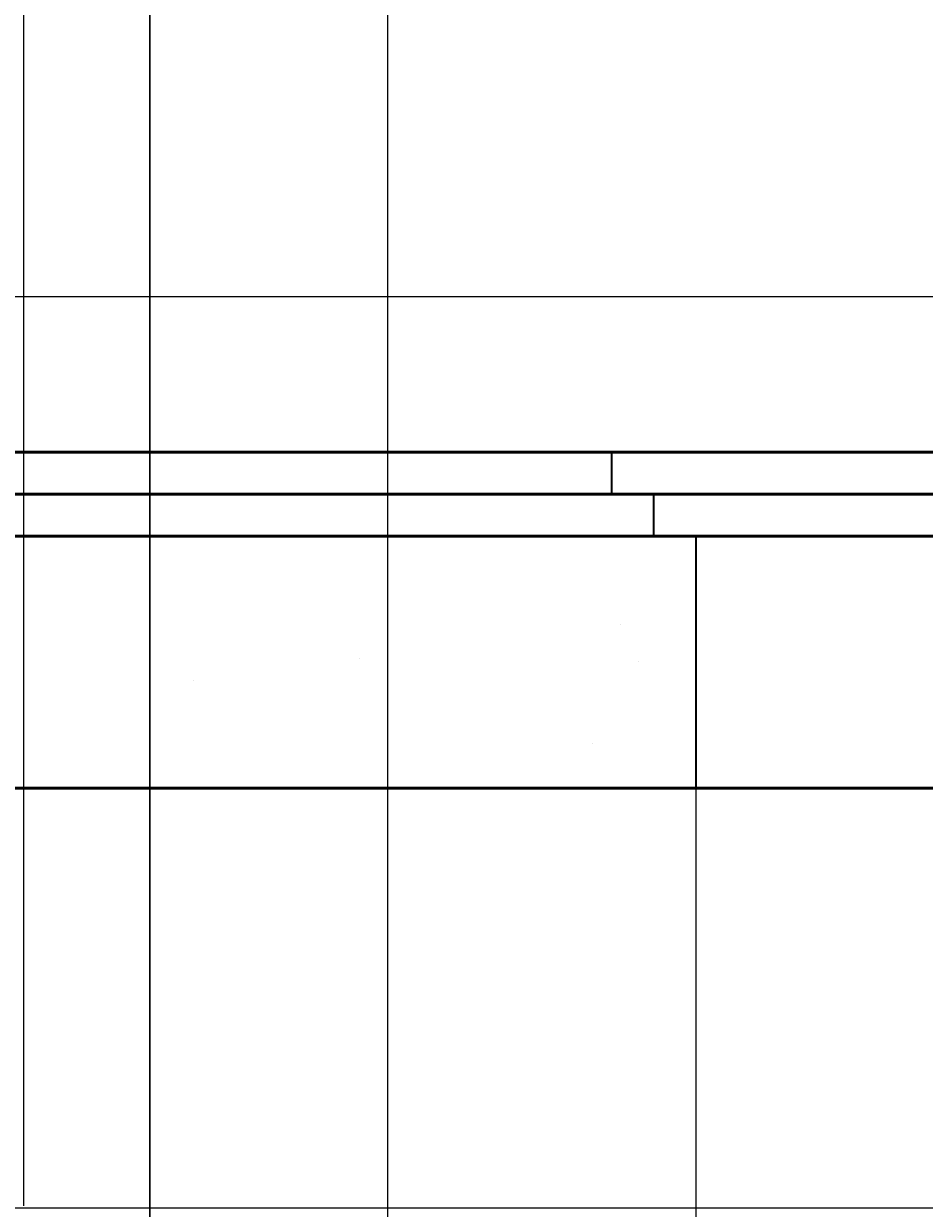
# Model space of a CAD drawing. Units: inches. Extents: x 2812 to 3051, y 1398 to 1659.
# Tile 23 of 65: x 2880 to 2902, y 1472 to 1500. Entities that reach past the tile are written whole.
import ezdxf

# ---------------------------------------------------------------- set-up
doc = ezdxf.new("R2010")
doc.units = ezdxf.units.IN
for name, color, linetype, lineweight in [('A-ANNO-DIMS', 2, 'Continuous', 18), ('S-CONC', 7, 'Continuous', 50), ('S-CONC-PATT', 8, 'Continuous', 18), ('S-CONC-SLAB', 7, 'Continuous', 35)]:
    doc.layers.add(name, color=color, linetype=linetype, lineweight=lineweight)
doc.styles.get("Standard").update_dxf_attribs({"font": 'arial.ttf'})
doc.dimstyles.get("Standard").update_dxf_attribs({"dimtxt": 0.18, "dimasz": 0.18, "dimexe": 0.18, "dimexo": 0.0625, "dimgap": 0.09, "dimtad": 0, "dimtih": 1, "dimtoh": 1, "dimdec": 4, "dimzin": 0, "dimdsep": 46, "dimtxsty": 'Standard', "dimcen": 0.09, "dimadec": 0, "dimazin": 0, "dimtfac": 1, "dimtdec": 4, "dimtofl": 0, "dimtmove": 0, "dimatfit": 3, "dimfxl": 1, "dimtolj": 1, "dimtzin": 0, "dimarcsym": 0})

# ---------------------------------------------------------------- blocks, each defined once
blk = doc.blocks.new('COVER-SLAB-PLAN')
for p, q in [((2, 7), (2, 8)), ((1, 6), (1, 7)), ((1, 7), (2, 7)), ((0, 6), (0, 0)), ((0, 6), (1, 6))]:
    blk.add_line(p, q)
blk = doc.blocks.new('*D29')
at = {"layer": 'A-ANNO-DIMS', "color": 0, "lineweight": -2, "transparency": 16777216}
for p, q in [((2910.742, 1598.757), (2910.742, 1397.505)), ((2883.385, 1559.757), (2883.385, 1397.505)), ((2883.565, 1397.685), (2896.598, 1397.685)), ((2910.562, 1397.685), (2897.528, 1397.685))]:
    blk.add_line(p, q, dxfattribs=at)
at = {"layer": 'A-ANNO-DIMS', "color": 0, "transparency": 16777216}
for points in [[(2883.565, 1397.715), (2883.565, 1397.655), (2883.385, 1397.685)], [(2910.562, 1397.715), (2910.562, 1397.655), (2910.742, 1397.685)]]:
    blk.add_solid(points, dxfattribs=at)
at = {"layer": 'Defpoints', "color": 0, "transparency": 16777216}
for p in [(2910.742, 1598.82), (2883.385, 1559.82), (2910.742, 1397.685)]:
    blk.add_point(p, dxfattribs=at)
at = {"layer": 'A-ANNO-DIMS', "color": 0, "transparency": 16777216, "insert": (2897.063, 1397.685), "char_height": 0.18, "attachment_point": 5}
blk.add_mtext('\\A1;27.357', dxfattribs=at)
blk = doc.blocks.new('*D44')
at = {"layer": 'A-ANNO-DIMS', "color": 0, "lineweight": -2, "transparency": 16777216}
for p, q in [((2850.748, 1487.973), (2850.748, 1397.505)), ((2896.385, 1487.973), (2896.385, 1397.505)), ((2850.928, 1397.685), (2873.17, 1397.685)), ((2896.205, 1397.685), (2873.964, 1397.685))]:
    blk.add_line(p, q, dxfattribs=at)
at = {"layer": 'A-ANNO-DIMS', "color": 0, "transparency": 16777216}
for points in [[(2850.928, 1397.715), (2850.928, 1397.655), (2850.748, 1397.685)], [(2896.205, 1397.715), (2896.205, 1397.655), (2896.385, 1397.685)]]:
    blk.add_solid(points, dxfattribs=at)
at = {"layer": 'Defpoints', "color": 0, "transparency": 16777216}
for p in [(2850.748, 1488.035), (2896.385, 1488.035), (2896.385, 1397.685)]:
    blk.add_point(p, dxfattribs=at)
at = {"layer": 'A-ANNO-DIMS', "color": 0, "transparency": 16777216, "insert": (2873.567, 1397.685), "char_height": 0.18, "attachment_point": 5}
blk.add_mtext('\\A1;45.64', dxfattribs=at)
blk = doc.blocks.new('*D45')
at = {"layer": 'A-ANNO-DIMS', "color": 0, "lineweight": -2, "transparency": 16777216}
for p, q in [((2896.385, 1487.973), (2896.385, 1397.505)), ((2941.385, 1487.973), (2941.385, 1397.505)), ((2896.565, 1397.685), (2918.662, 1397.685)), ((2941.205, 1397.685), (2919.108, 1397.685))]:
    blk.add_line(p, q, dxfattribs=at)
at = {"layer": 'A-ANNO-DIMS', "color": 0, "transparency": 16777216}
for points in [[(2896.565, 1397.715), (2896.565, 1397.655), (2896.385, 1397.685)], [(2941.205, 1397.715), (2941.205, 1397.655), (2941.385, 1397.685)]]:
    blk.add_solid(points, dxfattribs=at)
at = {"layer": 'Defpoints', "color": 0, "transparency": 16777216}
for p in [(2896.385, 1488.035), (2941.385, 1488.035), (2941.385, 1397.685)]:
    blk.add_point(p, dxfattribs=at)
at = {"layer": 'A-ANNO-DIMS', "color": 0, "transparency": 16777216, "insert": (2918.885, 1397.685), "char_height": 0.18, "attachment_point": 5}
blk.add_mtext('\\A1;45', dxfattribs=at)
blk = doc.blocks.new('*D55')
at = {"layer": 'A-ANNO-DIMS', "color": 0, "lineweight": -2, "transparency": 16777216}
for p, q in [((2850.811, 1493.738), (3051.178, 1493.738)), ((3050.998, 1493.558), (3050.998, 1491.069)), ((3050.998, 1488.215), (3050.998, 1490.705)), ((2850.811, 1488.035), (3051.178, 1488.035))]:
    blk.add_line(p, q, dxfattribs=at)
at = {"layer": 'A-ANNO-DIMS', "color": 0, "transparency": 16777216}
for points in [[(3050.968, 1493.558), (3051.028, 1493.558), (3050.998, 1493.738)], [(3050.968, 1488.215), (3051.028, 1488.215), (3050.998, 1488.035)]]:
    blk.add_solid(points, dxfattribs=at)
at = {"layer": 'Defpoints', "color": 0, "transparency": 16777216}
for p in [(2850.748, 1493.738), (3050.998, 1493.738), (2850.748, 1488.035)]:
    blk.add_point(p, dxfattribs=at)
at = {"layer": 'A-ANNO-DIMS', "color": 0, "transparency": 16777216, "insert": (3050.998, 1490.887), "char_height": 0.18, "attachment_point": 5}
blk.add_mtext('\\A1;5.703', dxfattribs=at)
blk = doc.blocks.new('*D58')
at = {"layer": 'A-ANNO-DIMS', "color": 0, "lineweight": -2, "transparency": 16777216}
for p, q in [((2880.385, 1472.098), (2880.385, 1659.35)), ((2883.385, 1472.098), (2883.385, 1659.35)), ((2880.565, 1659.17), (2881.736, 1659.17)), ((2883.205, 1659.17), (2882.034, 1659.17))]:
    blk.add_line(p, q, dxfattribs=at)
at = {"layer": 'A-ANNO-DIMS', "color": 0, "transparency": 16777216}
for points in [[(2880.565, 1659.2), (2880.565, 1659.14), (2880.385, 1659.17)], [(2883.205, 1659.2), (2883.205, 1659.14), (2883.385, 1659.17)]]:
    blk.add_solid(points, dxfattribs=at)
at = {"layer": 'Defpoints', "color": 0, "transparency": 16777216}
for p in [(2883.385, 1659.17), (2880.385, 1472.035), (2883.385, 1472.035)]:
    blk.add_point(p, dxfattribs=at)
at = {"layer": 'A-ANNO-DIMS', "color": 0, "transparency": 16777216, "insert": (2881.885, 1659.17), "char_height": 0.18, "attachment_point": 5}
blk.add_mtext('\\A1;3', dxfattribs=at)
blk = doc.blocks.new('*D59')
at = {"layer": 'A-ANNO-DIMS', "color": 0, "lineweight": -2, "transparency": 16777216}
for p, q in [((2883.385, 1452.098), (2883.385, 1659.35)), ((2889.058, 1467.465), (2889.058, 1659.35)), ((2883.565, 1659.17), (2885.828, 1659.17)), ((2888.878, 1659.17), (2886.615, 1659.17))]:
    blk.add_line(p, q, dxfattribs=at)
at = {"layer": 'A-ANNO-DIMS', "color": 0, "transparency": 16777216}
for points in [[(2883.565, 1659.2), (2883.565, 1659.14), (2883.385, 1659.17)], [(2888.878, 1659.2), (2888.878, 1659.14), (2889.058, 1659.17)]]:
    blk.add_solid(points, dxfattribs=at)
at = {"layer": 'Defpoints', "color": 0, "transparency": 16777216}
for p in [(2889.058, 1659.17), (2889.058, 1467.402), (2883.385, 1452.035)]:
    blk.add_point(p, dxfattribs=at)
at = {"layer": 'A-ANNO-DIMS', "color": 0, "transparency": 16777216, "insert": (2886.221, 1659.17), "char_height": 0.18, "attachment_point": 5}
blk.add_mtext('\\A1;5.673', dxfattribs=at)
blk = doc.blocks.new('*D77')
at = {"layer": 'A-ANNO-DIMS', "color": 0, "lineweight": -2, "transparency": 16777216}
for p, q in [((2961.322, 1472.035), (2811.806, 1472.035)), ((2811.986, 1471.855), (2811.986, 1461.436)), ((2811.986, 1450.654), (2811.986, 1461.073)), ((2963.812, 1450.474), (2811.806, 1450.474))]:
    blk.add_line(p, q, dxfattribs=at)
at = {"layer": 'A-ANNO-DIMS', "color": 0, "transparency": 16777216}
for points in [[(2811.956, 1471.855), (2812.016, 1471.855), (2811.986, 1472.035)], [(2811.956, 1450.654), (2812.016, 1450.654), (2811.986, 1450.474)]]:
    blk.add_solid(points, dxfattribs=at)
at = {"layer": 'Defpoints', "color": 0, "transparency": 16777216}
for p in [(2811.986, 1472.035), (2961.385, 1472.035), (2963.874, 1450.474)]:
    blk.add_point(p, dxfattribs=at)
at = {"layer": 'A-ANNO-DIMS', "color": 0, "transparency": 16777216, "insert": (2811.986, 1461.255), "char_height": 0.18, "attachment_point": 5}
blk.add_mtext('\\A1;21.56', dxfattribs=at)

msp = doc.modelspace()

# ---------------------------------------------------------------- hatches: boundary and pattern name
at = {"layer": 'S-CONC-PATT'}
h = msp.add_hatch(dxfattribs=at)
h.set_pattern_fill('AR-SAND', color=256, scale=0.3)
h.paths.add_polyline_path([(3036.3849, 1416.0354), (3027.3849, 1416.0354), (2826.3849, 1416.0354), (2826.3849, 1410.0354), (2835.3849, 1410.0354), (3036.3849, 1410.0354)])
h.paths.add_polyline_path([(2970.3849, 1488.0354), (2969.3849, 1488.0354), (2941.3849, 1488.0354), (2941.3849, 1482.0354), (2970.3849, 1482.0354)])
h.paths.add_polyline_path([(3036.3849, 1488.0354), (3035.3849, 1488.0354), (3006.3849, 1488.0354), (3006.3849, 1482.0354), (3027.3849, 1482.0354), (3036.3849, 1482.0354)])
h.paths.add_polyline_path([(3034.3849, 1490.0354), (3008.3849, 1490.0354), (3008.3849, 1489.0354), (3034.3849, 1489.0354)])
h.paths.add_polyline_path([(3035.3849, 1489.0354), (3034.3849, 1489.0354), (3007.3849, 1489.0354), (3007.3849, 1488.0354), (3035.3849, 1488.0354)])
h.paths.add_polyline_path([(2968.3849, 1490.0354), (2943.3849, 1490.0354), (2943.3849, 1489.0354), (2968.3849, 1489.0354)])
h.paths.add_polyline_path([(2969.3849, 1489.0354), (2968.3849, 1489.0354), (2942.3849, 1489.0354), (2942.3849, 1488.0354), (2969.3849, 1488.0354)])
h.paths.add_polyline_path([(2896.3849, 1488.0354), (2826.3849, 1488.0354), (2826.3849, 1482.0354), (2896.3849, 1482.0354)])
h.paths.add_polyline_path([(2895.3849, 1489.0354), (2894.3849, 1489.0354), (2827.3849, 1489.0354), (2827.3849, 1488.0354), (2895.3849, 1488.0354)])
h.paths.add_polyline_path([(2894.3849, 1490.0354), (2828.3849, 1490.0354), (2828.3849, 1489.0354), (2894.3849, 1489.0354)])
h = msp.add_hatch(dxfattribs=at)
h.set_pattern_fill('AR-CONC', color=256, scale=0.3)
h.paths.add_polyline_path([(2896.3849, 1488.0354), (2826.3849, 1488.0354), (2826.3849, 1482.0354), (2896.3849, 1482.0354)])
h.paths.add_polyline_path([(2970.3849, 1488.0354), (2941.3849, 1488.0354), (2941.3849, 1482.0354), (2970.3849, 1482.0354)])
h.paths.add_polyline_path([(2968.3849, 1490.0354), (2943.3849, 1490.0354), (2943.3849, 1489.0354), (2968.3849, 1489.0354)])
h.paths.add_polyline_path([(2969.3849, 1489.0354), (2968.3849, 1489.0354), (2943.3849, 1489.0354), (2942.3849, 1489.0354), (2942.3849, 1488.0354), (2969.3849, 1488.0354)])
h.paths.add_polyline_path([(3036.3849, 1488.0354), (3035.3849, 1488.0354), (3006.3849, 1488.0354), (3006.3849, 1482.0354), (3027.3849, 1482.0354), (3036.3849, 1482.0354)])
h.paths.add_polyline_path([(3035.3849, 1489.0354), (3034.3849, 1489.0354), (3007.3849, 1489.0354), (3007.3849, 1488.0354), (3035.3849, 1488.0354)])
h.paths.add_polyline_path([(3034.3849, 1490.0354), (3008.3849, 1490.0354), (3008.3849, 1489.0354), (3034.3849, 1489.0354)])
h.paths.add_polyline_path([(2895.3849, 1489.0354), (2894.3849, 1489.0354), (2827.3849, 1489.0354), (2827.3849, 1488.0354), (2895.3849, 1488.0354)])
h.paths.add_polyline_path([(2894.3849, 1490.0354), (2828.3849, 1490.0354), (2828.3849, 1489.0354), (2894.3849, 1489.0354)])

# ---------------------------------------------------------------- linework, layer by layer
at = {"layer": 'S-CONC'}
for p, q in [((3034.3849, 1490.0354), (2850.7485, 1490.0354)), ((2850.7485, 1489.0354), (3035.3849, 1489.0354)), ((2850.7485, 1488.0354), (3036.3849, 1488.0354)), ((2850.7485, 1482.0354), (3027.3849, 1482.0354))]:
    msp.add_line(p, q, dxfattribs=at)

# ---------------------------------------------------------------- block references
at = {"layer": 'S-CONC-SLAB', "extrusion": (0, 0, -1), "zscale": -1}
msp.add_blockref('COVER-SLAB-PLAN', (-2896.3848, 1482.035), dxfattribs=at)

# ---------------------------------------------------------------- dimensions: what is measured, and where the dimension line sits
at = {"layer": 'A-ANNO-DIMS'}
for base, p1, p2, override, picture, middle in [((2883.3849, 1659.17), (2880.3849, 1472.0354), (2883.3849, 1472.0354), {"dimdec": 0, "dimlfac": 1, "dimrnd": 0, "dimzin": 0, "dimdsep": 46, "dimlunit": 2}, '*D58', (2881.8849, 1659.17)), ((2889.0577, 1659.17), (2883.3849, 1452.0354), (2889.0577, 1467.4024), {"dimdec": 3, "dimlfac": 1, "dimrnd": 0, "dimzin": 0, "dimdsep": 46, "dimlunit": 2}, '*D59', (2886.2213, 1659.17)), ((2910.7415, 1397.6854), (2883.3849, 1559.82), (2910.7415, 1598.82), {"dimdec": 3, "dimlfac": 1, "dimrnd": 0, "dimzin": 0, "dimdsep": 46, "dimlunit": 2}, '*D29', (2897.0632, 1397.6854)), ((2896.3849, 1397.6854), (2850.7485, 1488.0354), (2896.3849, 1488.0354), {"dimdec": 2, "dimlfac": 1, "dimrnd": 0, "dimzin": 0, "dimdsep": 46, "dimlunit": 2}, '*D44', (2873.5667, 1397.6854)), ((2941.3849, 1397.6854), (2896.3849, 1488.0354), (2941.3849, 1488.0354), {"dimdec": 0, "dimlfac": 1, "dimrnd": 0, "dimzin": 0, "dimdsep": 46, "dimlunit": 2}, '*D45', (2918.8849, 1397.6854))]:
    dim = msp.add_linear_dim(base=base, p1=p1, p2=p2, dimstyle='Standard', override=override, dxfattribs=at)
    dim.commit()
    dim.dimension.update_dxf_attribs({"geometry": picture, "text_midpoint": middle})
for base, p1, p2, override, picture, middle in [((3050.998, 1493.7383), (2850.7485, 1488.0354), (2850.7485, 1493.7383), {"dimdec": 3, "dimlfac": 1, "dimrnd": 0, "dimzin": 0, "dimdsep": 46, "dimlunit": 2}, '*D55', (3050.998, 1490.8868)), ((2811.9855, 1472.0354), (2963.8741, 1450.4738), (2961.3849, 1472.0354), {"dimdec": 2, "dimlfac": 1, "dimrnd": 0, "dimzin": 0, "dimdsep": 46, "dimlunit": 2}, '*D77', (2811.9855, 1461.2546))]:
    dim = msp.add_linear_dim(base=base, p1=p1, p2=p2, angle=90, dimstyle='Standard', override=override, dxfattribs=at)
    dim.commit()
    dim.dimension.update_dxf_attribs({"geometry": picture, "text_midpoint": middle})

doc.saveas('drawing.dxf')
